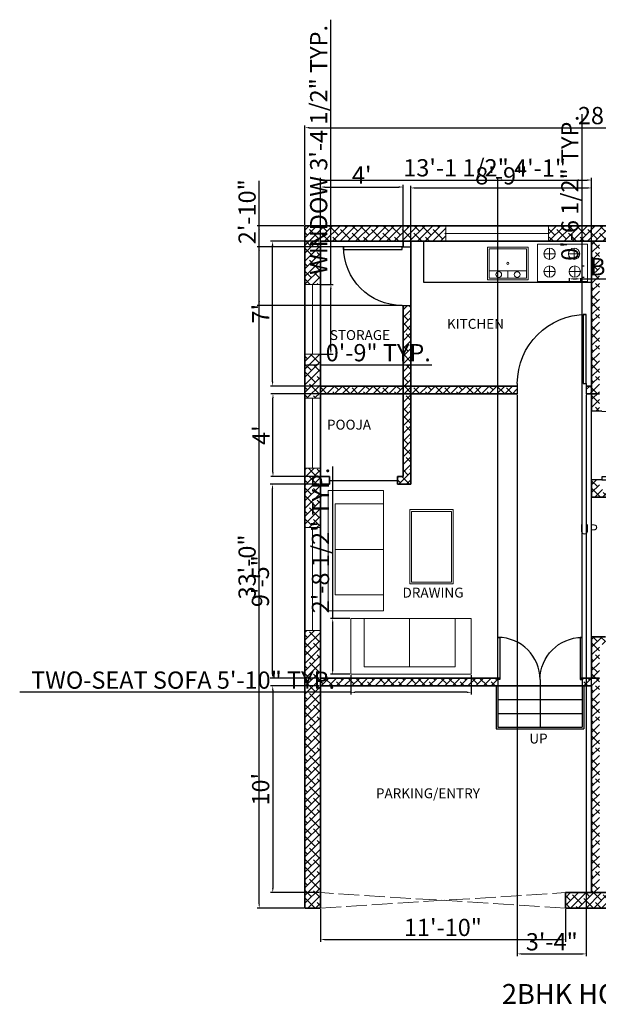
# Model space of a CAD drawing. Units: inches. Extents: x 1501 to 2163, y 1105 to 1729.
# Tile 1 of 2: x 1501 to 1837, y 1105 to 1676. Entities that reach past the tile are written whole.
import ezdxf

# ---------------------------------------------------------------- set-up
doc = ezdxf.new("R2010")
doc.units = ezdxf.units.IN
doc.linetypes.add('ACAD_ISO02W100', pattern=[15, 12, -3])
for name, color, linetype, lineweight in [('A-ANNO-DIMS', 2, 'Continuous', 18), ('A-ANNO-TEXT', 7, 'Continuous', 18), ('A-AREA-IDEN', 7, 'Continuous', 18), ('A-DOOR', 3, 'Continuous', 25), ('A-DOOR-OPEN', 3, 'ACAD_ISO02W100', 18), ('A-EQPM', 9, 'Continuous', 18), ('A-FLOR-CASE', 8, 'Continuous', 25), ('A-FLOR-FIXT', 9, 'Continuous', 18), ('A-FLOR-STRS', 7, 'Continuous', 25), ('A-GLAZ', 4, 'Continuous', 18), ('A-WALL', 7, 'Continuous', 35), ('A-WALL-PATT', 252, 'Continuous', 13), ('fur', 130, 'Continuous', 18)]:
    doc.layers.add(name, color=color, linetype=linetype, lineweight=lineweight)
doc.styles.get("Standard").update_dxf_attribs({"font": 'arial.ttf'})
doc.dimstyles.new('ISO-25', dxfattribs={"dimtxt": 10, "dimasz": 2.5, "dimexe": 1.25, "dimexo": 0.625, "dimtad": 1, "dimdec": 0, "dimlunit": 4, "dimtxsty": 'Standard', "dimcen": 2.5, "dimadec": 0, "dimazin": 0, "dimtfac": 1, "dimtdec": 0, "dimtmove": 0, "dimatfit": 3, "dimfxl": 1, "dimarcsym": 0})

# ---------------------------------------------------------------- blocks, each defined once
blk = doc.blocks.new('*U2')
for p, q in [((0, 0), (0, -6)), ((40, 0), (40, -6))]:
    blk.add_line(p, q)
blk.add_lwpolyline([(0, 0), (0, 40), (1.75, 40), (1.75, 0)], close=True)
blk.add_arc((0, 0), 40, 0, 90)
blk = doc.blocks.new('*D12')
at = {"layer": 'A-ANNO-DIMS', "color": 0, "lineweight": -2, "transparency": 16777216}
for p, q in [((1666.55, 1557.41), (1666.55, 1614.95)), ((1669.05, 1613.7), (2000.05, 1613.7)), ((2002.55, 1557.41), (2002.55, 1614.95))]:
    blk.add_line(p, q, dxfattribs=at)
at = {"layer": 'A-ANNO-DIMS', "color": 0, "lineweight": 100, "transparency": 16777216}
for points in [[(1669.05, 1614.12), (1669.05, 1613.29), (1666.55, 1613.7)], [(2000.05, 1614.12), (2000.05, 1613.29), (2002.55, 1613.7)]]:
    blk.add_solid(points, dxfattribs=at)
at = {"layer": 'Defpoints', "color": 0, "lineweight": 100, "transparency": 16777216}
for p in [(2002.55, 1613.7), (1666.55, 1556.78), (2002.55, 1556.78)]:
    blk.add_point(p, dxfattribs=at)
at = {"layer": 'A-ANNO-DIMS', "color": 0, "transparency": 16777216, "insert": (1834.55, 1619.44), "char_height": 10, "attachment_point": 5}
blk.add_mtext("28'", dxfattribs=at)
blk = doc.blocks.new('*D13')
at = {"layer": 'A-ANNO-DIMS', "color": 0, "lineweight": -2, "transparency": 16777216}
for p, q in [((1675.55, 1548.41), (1675.55, 1580.52)), ((1678.05, 1579.27), (1721.05, 1579.27)), ((1723.55, 1548.41), (1723.55, 1580.52))]:
    blk.add_line(p, q, dxfattribs=at)
at = {"layer": 'A-ANNO-DIMS', "color": 0, "lineweight": 100, "transparency": 16777216}
for points in [[(1678.05, 1579.69), (1678.05, 1578.85), (1675.55, 1579.27)], [(1721.05, 1579.69), (1721.05, 1578.85), (1723.55, 1579.27)]]:
    blk.add_solid(points, dxfattribs=at)
at = {"layer": 'Defpoints', "color": 0, "lineweight": 100, "transparency": 16777216}
for p in [(1723.55, 1579.27), (1675.55, 1547.78), (1723.55, 1547.78)]:
    blk.add_point(p, dxfattribs=at)
at = {"layer": 'A-ANNO-DIMS', "color": 0, "transparency": 16777216, "insert": (1699.55, 1584.89), "char_height": 10, "attachment_point": 5}
blk.add_mtext("4'", dxfattribs=at)
blk = doc.blocks.new('*D14')
at = {"layer": 'A-ANNO-DIMS', "color": 0, "lineweight": -2, "transparency": 16777216}
for p, q in [((1728.05, 1548.41), (1728.05, 1579.99)), ((1730.55, 1578.74), (1830.55, 1578.74)), ((1833.05, 1548.41), (1833.05, 1579.99))]:
    blk.add_line(p, q, dxfattribs=at)
at = {"layer": 'A-ANNO-DIMS', "color": 0, "lineweight": 100, "transparency": 16777216}
for points in [[(1730.55, 1579.15), (1730.55, 1578.32), (1728.05, 1578.74)], [(1830.55, 1579.15), (1830.55, 1578.32), (1833.05, 1578.74)]]:
    blk.add_solid(points, dxfattribs=at)
at = {"layer": 'Defpoints', "color": 0, "lineweight": 100, "transparency": 16777216}
for p in [(1833.05, 1578.74), (1728.05, 1547.78), (1833.05, 1547.78)]:
    blk.add_point(p, dxfattribs=at)
at = {"layer": 'A-ANNO-DIMS', "color": 0, "transparency": 16777216, "insert": (1780.55, 1584.47), "char_height": 10, "attachment_point": 5}
blk.add_mtext('8\'-9"', dxfattribs=at)
blk = doc.blocks.new('*D20')
at = {"layer": 'A-ANNO-DIMS', "color": 0, "lineweight": -2, "transparency": 16777216}
for p, q in [((1675.55, 1160.16), (1675.55, 1141.32)), ((1817.84, 1160.16), (1817.84, 1141.32)), ((1678.05, 1142.57), (1815.34, 1142.57))]:
    blk.add_line(p, q, dxfattribs=at)
at = {"layer": 'A-ANNO-DIMS', "color": 0, "lineweight": 100, "transparency": 16777216}
for points in [[(1678.05, 1142.98), (1678.05, 1142.15), (1675.55, 1142.57)], [(1815.34, 1142.98), (1815.34, 1142.15), (1817.84, 1142.57)]]:
    blk.add_solid(points, dxfattribs=at)
at = {"layer": 'Defpoints', "color": 0, "lineweight": 100, "transparency": 16777216}
for p in [(1675.55, 1160.78), (1817.84, 1160.78), (1817.84, 1142.57)]:
    blk.add_point(p, dxfattribs=at)
at = {"layer": 'A-ANNO-DIMS', "color": 0, "transparency": 16777216, "insert": (1746.69, 1148.3), "char_height": 10, "attachment_point": 5}
blk.add_mtext('11\'-10"', dxfattribs=at)
blk = doc.blocks.new('*D21')
at = {"layer": 'A-ANNO-DIMS', "color": 0, "lineweight": -2, "transparency": 16777216}
for p, q in [((1674.93, 1289.78), (1646.64, 1289.78)), ((1647.89, 1287.28), (1647.89, 1172.28)), ((1674.93, 1169.78), (1646.64, 1169.78))]:
    blk.add_line(p, q, dxfattribs=at)
at = {"layer": 'A-ANNO-DIMS', "color": 0, "lineweight": 100, "transparency": 16777216}
for points in [[(1647.47, 1287.28), (1648.3, 1287.28), (1647.89, 1289.78)], [(1647.47, 1172.28), (1648.3, 1172.28), (1647.89, 1169.78)]]:
    blk.add_solid(points, dxfattribs=at)
at = {"layer": 'Defpoints', "color": 0, "lineweight": 100, "transparency": 16777216}
for p in [(1675.55, 1289.78), (1647.89, 1169.78), (1675.55, 1169.78)]:
    blk.add_point(p, dxfattribs=at)
at = {"layer": 'A-ANNO-DIMS', "color": 0, "transparency": 16777216, "insert": (1642.15, 1229.78), "char_height": 10, "attachment_point": 5, "rotation": 90}
blk.add_mtext("10'", dxfattribs=at)
blk = doc.blocks.new('*D22')
at = {"layer": 'A-ANNO-DIMS', "color": 0, "lineweight": -2, "transparency": 16777216}
for p, q in [((1674.93, 1406.78), (1646.47, 1406.78)), ((1647.72, 1296.78), (1647.72, 1404.28)), ((1674.93, 1294.28), (1646.47, 1294.28))]:
    blk.add_line(p, q, dxfattribs=at)
at = {"layer": 'A-ANNO-DIMS', "color": 0, "lineweight": 100, "transparency": 16777216}
for points in [[(1647.31, 1404.28), (1648.14, 1404.28), (1647.72, 1406.78)], [(1647.31, 1296.78), (1648.14, 1296.78), (1647.72, 1294.28)]]:
    blk.add_solid(points, dxfattribs=at)
at = {"layer": 'Defpoints', "color": 0, "lineweight": 100, "transparency": 16777216}
for p in [(1647.72, 1406.78), (1675.55, 1406.78), (1675.55, 1294.28)]:
    blk.add_point(p, dxfattribs=at)
at = {"layer": 'A-ANNO-DIMS', "color": 0, "transparency": 16777216, "insert": (1641.99, 1350.53), "char_height": 10, "attachment_point": 5, "rotation": 90}
blk.add_mtext('9\'-5"', dxfattribs=at)
blk = doc.blocks.new('*D23')
at = {"layer": 'A-ANNO-DIMS', "color": 0, "lineweight": -2, "transparency": 16777216}
for p, q in [((1674.93, 1459.28), (1646.75, 1459.28)), ((1648, 1413.78), (1648, 1456.78)), ((1674.93, 1411.28), (1646.75, 1411.28))]:
    blk.add_line(p, q, dxfattribs=at)
at = {"layer": 'A-ANNO-DIMS', "color": 0, "lineweight": 100, "transparency": 16777216}
for points in [[(1647.59, 1456.78), (1648.42, 1456.78), (1648, 1459.28)], [(1647.59, 1413.78), (1648.42, 1413.78), (1648, 1411.28)]]:
    blk.add_solid(points, dxfattribs=at)
at = {"layer": 'Defpoints', "color": 0, "lineweight": 100, "transparency": 16777216}
for p in [(1648, 1459.28), (1675.55, 1459.28), (1675.55, 1411.28)]:
    blk.add_point(p, dxfattribs=at)
at = {"layer": 'A-ANNO-DIMS', "color": 0, "transparency": 16777216, "insert": (1642.38, 1435.28), "char_height": 10, "attachment_point": 5, "rotation": 90}
blk.add_mtext("4'", dxfattribs=at)
blk = doc.blocks.new('*D24')
at = {"layer": 'A-ANNO-DIMS', "color": 0, "lineweight": -2, "transparency": 16777216}
for p, q in [((1674.93, 1547.78), (1646.55, 1547.78)), ((1647.8, 1466.28), (1647.8, 1545.28)), ((1674.93, 1463.78), (1646.55, 1463.78))]:
    blk.add_line(p, q, dxfattribs=at)
at = {"layer": 'A-ANNO-DIMS', "color": 0, "lineweight": 100, "transparency": 16777216}
for points in [[(1647.38, 1545.28), (1648.21, 1545.28), (1647.8, 1547.78)], [(1647.38, 1466.28), (1648.21, 1466.28), (1647.8, 1463.78)]]:
    blk.add_solid(points, dxfattribs=at)
at = {"layer": 'Defpoints', "color": 0, "lineweight": 100, "transparency": 16777216}
for p in [(1647.8, 1547.78), (1675.55, 1547.78), (1675.55, 1463.78)]:
    blk.add_point(p, dxfattribs=at)
at = {"layer": 'A-ANNO-DIMS', "color": 0, "transparency": 16777216, "insert": (1642.17, 1505.78), "char_height": 10, "attachment_point": 5, "rotation": 90}
blk.add_mtext("7'", dxfattribs=at)
blk = doc.blocks.new('WIN-60IN')
blk.add_line((0, 4.5), (59.67, 4.5))
blk.add_lwpolyline([(0, 9), (59.67, 9), (59.67, 0), (0, 0)], close=True)
blk = doc.blocks.new('WIN-41IN')
blk.add_line((4.5, 0), (4.5, 40.59))
blk.add_lwpolyline([(0, 0), (9, 0), (9, 40.59), (0, 40.59)], close=True)
blk = doc.blocks.new('SOFA-TWO-SEAT')
for p, q in [((32.31, 69.96), (0, 69.96)), ((0, 69.96), (0, 0)), ((32.31, 62.16), (32.31, 69.96)), ((4.25, 35.75), (32.31, 35.75)), ((32.31, 0), (32.31, 9.35)), ((0, 0), (32.31, 0))]:
    blk.add_line(p, q)
blk.add_lwpolyline([(4.25, 62.16), (32.31, 62.16), (32.31, 9.35), (4.25, 9.35)], close=True)
blk = doc.blocks.new('COOKTOP-BURNER')
for p, q in [((3.26, 6.53), (3.26, 0)), ((6.53, 3.27), (0, 3.27)), ((3.26, 0), (3.26, 3.27)), ((3.26, 3.27), (6.53, 3.27))]:
    blk.add_line(p, q)
blk.add_circle((3.26, 3.27), 3.26)
blk = doc.blocks.new('*D34')
at = {"layer": 'A-ANNO-DIMS', "color": 0, "lineweight": -2, "transparency": 16777216}
for p, q in [((1681.64, 1522.79), (1681.64, 1676.38)), ((1676.18, 1522.79), (1682.89, 1522.79)), ((1681.64, 1484.69), (1681.64, 1520.29)), ((1676.18, 1482.19), (1682.89, 1482.19))]:
    blk.add_line(p, q, dxfattribs=at)
at = {"layer": 'A-ANNO-DIMS', "color": 0, "lineweight": 100, "transparency": 16777216}
for points in [[(1681.22, 1520.29), (1682.06, 1520.29), (1681.64, 1522.79)], [(1681.22, 1484.69), (1682.06, 1484.69), (1681.64, 1482.19)]]:
    blk.add_solid(points, dxfattribs=at)
at = {"layer": 'Defpoints', "color": 0, "lineweight": 100, "transparency": 16777216}
for p in [(1675.55, 1522.79), (1681.64, 1522.79), (1675.55, 1482.19)]:
    blk.add_point(p, dxfattribs=at)
at = {"layer": 'A-ANNO-DIMS', "color": 0, "transparency": 16777216, "insert": (1675.84, 1600.83), "char_height": 10, "attachment_point": 5, "rotation": 90}
blk.add_mtext('WINDOW 3\'-4 1/2" TYP.', dxfattribs=at)
blk = doc.blocks.new('*D35')
at = {"layer": 'A-ANNO-DIMS', "color": 0, "lineweight": -2, "transparency": 16777216}
for p, q in [((1666.55, 1481.57), (1666.55, 1474.86)), ((1675.55, 1481.57), (1675.55, 1474.86)), ((1669.05, 1476.11), (1673.05, 1476.11)), ((1675.55, 1476.11), (1740.26, 1476.11))]:
    blk.add_line(p, q, dxfattribs=at)
at = {"layer": 'A-ANNO-DIMS', "color": 0, "lineweight": 100, "transparency": 16777216}
for points in [[(1669.05, 1476.52), (1669.05, 1475.69), (1666.55, 1476.11)], [(1673.05, 1476.52), (1673.05, 1475.69), (1675.55, 1476.11)]]:
    blk.add_solid(points, dxfattribs=at)
at = {"layer": 'Defpoints', "color": 0, "lineweight": 100, "transparency": 16777216}
for p in [(1666.55, 1482.19), (1675.55, 1482.19), (1675.55, 1476.11)]:
    blk.add_point(p, dxfattribs=at)
at = {"layer": 'A-ANNO-DIMS', "color": 0, "transparency": 16777216, "insert": (1709.15, 1481.84), "char_height": 10, "attachment_point": 5}
blk.add_mtext('0\'-9" TYP.', dxfattribs=at)
blk = doc.blocks.new('*D36')
at = {"layer": 'A-ANNO-DIMS', "color": 0, "lineweight": -2, "transparency": 16777216}
for p, q in [((1693.17, 1295.9), (1693.17, 1284.78)), ((1763.13, 1295.9), (1763.13, 1284.78)), ((1693.17, 1286.03), (1500.92, 1286.03)), ((1760.63, 1286.03), (1695.67, 1286.03))]:
    blk.add_line(p, q, dxfattribs=at)
at = {"layer": 'A-ANNO-DIMS', "color": 0, "lineweight": 100, "transparency": 16777216}
for points in [[(1695.67, 1286.44), (1695.67, 1285.61), (1693.17, 1286.03)], [(1760.63, 1286.44), (1760.63, 1285.61), (1763.13, 1286.03)]]:
    blk.add_solid(points, dxfattribs=at)
at = {"layer": 'Defpoints', "color": 0, "lineweight": 100, "transparency": 16777216}
for p in [(1693.17, 1296.52), (1763.13, 1296.52), (1693.17, 1286.03)]:
    blk.add_point(p, dxfattribs=at)
at = {"layer": 'A-ANNO-DIMS', "color": 0, "transparency": 16777216, "insert": (1595.8, 1291.83), "char_height": 10, "attachment_point": 5}
blk.add_mtext('TWO-SEAT SOFA 5\'-10" TYP.', dxfattribs=at)
blk = doc.blocks.new('*D37')
at = {"layer": 'A-ANNO-DIMS', "color": 0, "lineweight": -2, "transparency": 16777216}
for p, q in [((1682.68, 1328.83), (1682.68, 1417.01)), ((1692.55, 1328.83), (1681.43, 1328.83)), ((1682.68, 1299.02), (1682.68, 1326.33)), ((1692.55, 1296.52), (1681.43, 1296.52))]:
    blk.add_line(p, q, dxfattribs=at)
at = {"layer": 'A-ANNO-DIMS', "color": 0, "lineweight": 100, "transparency": 16777216}
for points in [[(1682.26, 1326.33), (1683.1, 1326.33), (1682.68, 1328.83)], [(1682.26, 1299.02), (1683.1, 1299.02), (1682.68, 1296.52)]]:
    blk.add_solid(points, dxfattribs=at)
at = {"layer": 'Defpoints', "color": 0, "lineweight": 100, "transparency": 16777216}
for p in [(1682.68, 1328.83), (1693.17, 1328.83), (1693.17, 1296.52)]:
    blk.add_point(p, dxfattribs=at)
at = {"layer": 'A-ANNO-DIMS', "color": 0, "transparency": 16777216, "insert": (1676.88, 1374.17), "char_height": 10, "attachment_point": 5, "rotation": 90}
blk.add_mtext('2\'-8 1/2" TYP.', dxfattribs=at)
blk = doc.blocks.new('*D44')
at = {"layer": 'A-ANNO-DIMS', "color": 0, "lineweight": -2, "transparency": 16777216}
for p, q in [((1820, 1526.33), (1820, 1524.73)), ((1822.5, 1525.98), (1824.03, 1525.98)), ((1826.53, 1526.33), (1826.53, 1524.73)), ((1826.53, 1525.98), (1976.97, 1525.98))]:
    blk.add_line(p, q, dxfattribs=at)
at = {"layer": 'A-ANNO-DIMS', "color": 0, "lineweight": 100, "transparency": 16777216}
for points in [[(1822.5, 1526.39), (1822.5, 1525.56), (1820, 1525.98)], [(1824.03, 1526.39), (1824.03, 1525.56), (1826.53, 1525.98)]]:
    blk.add_solid(points, dxfattribs=at)
at = {"layer": 'Defpoints', "color": 0, "lineweight": 100, "transparency": 16777216}
for p in [(1820, 1526.95), (1826.53, 1526.95), (1826.53, 1525.98)]:
    blk.add_point(p, dxfattribs=at)
at = {"layer": 'A-ANNO-DIMS', "color": 0, "transparency": 16777216, "insert": (1903, 1531.77), "char_height": 10, "attachment_point": 5}
blk.add_mtext('BURNER 0\'-6 1/2" TYP.', dxfattribs=at)
blk = doc.blocks.new('*D45')
at = {"layer": 'A-ANNO-DIMS', "color": 0, "lineweight": -2, "transparency": 16777216}
for p, q in [((1827.51, 1533.48), (1827.51, 1621.49)), ((1827.16, 1533.48), (1828.76, 1533.48)), ((1827.16, 1526.95), (1828.76, 1526.95)), ((1827.51, 1529.45), (1827.51, 1530.98))]:
    blk.add_line(p, q, dxfattribs=at)
at = {"layer": 'A-ANNO-DIMS', "color": 0, "lineweight": 100, "transparency": 16777216}
for points in [[(1827.1, 1530.98), (1827.93, 1530.98), (1827.51, 1533.48)], [(1827.1, 1529.45), (1827.93, 1529.45), (1827.51, 1526.95)]]:
    blk.add_solid(points, dxfattribs=at)
at = {"layer": 'Defpoints', "color": 0, "lineweight": 100, "transparency": 16777216}
for p in [(1826.53, 1533.48), (1827.51, 1533.48), (1826.53, 1526.95)]:
    blk.add_point(p, dxfattribs=at)
at = {"layer": 'A-ANNO-DIMS', "color": 0, "transparency": 16777216, "insert": (1821.72, 1578.74), "char_height": 10, "attachment_point": 5, "rotation": 90}
blk.add_mtext('0\'-6 1/2" TYP.', dxfattribs=at)
blk = doc.blocks.new('*D46')
at = {"layer": 'A-ANNO-DIMS', "color": 0, "lineweight": -2, "transparency": 16777216}
for p, q in [((1665.93, 1556.78), (1638.75, 1556.78)), ((1640, 1163.28), (1640, 1554.28)), ((1665.93, 1160.78), (1638.75, 1160.78))]:
    blk.add_line(p, q, dxfattribs=at)
at = {"layer": 'A-ANNO-DIMS', "color": 0, "lineweight": 100, "transparency": 16777216}
for points in [[(1639.58, 1554.28), (1640.42, 1554.28), (1640, 1556.78)], [(1639.58, 1163.28), (1640.42, 1163.28), (1640, 1160.78)]]:
    blk.add_solid(points, dxfattribs=at)
at = {"layer": 'Defpoints', "color": 0, "lineweight": 100, "transparency": 16777216}
for p in [(1640, 1556.78), (1666.55, 1556.78), (1666.55, 1160.78)]:
    blk.add_point(p, dxfattribs=at)
at = {"layer": 'A-ANNO-DIMS', "color": 0, "transparency": 16777216, "insert": (1634.27, 1358.78), "char_height": 10, "attachment_point": 5, "rotation": 90}
blk.add_mtext('33\'-0"', dxfattribs=at)
blk = doc.blocks.new('*D47')
at = {"layer": 'A-ANNO-DIMS', "color": 0, "lineweight": -2, "transparency": 16777216}
for p, q in [((1778.68, 1294.07), (1778.68, 1584.58)), ((1781.18, 1583.33), (1825.03, 1583.33)), ((1827.53, 1294.07), (1827.53, 1584.58))]:
    blk.add_line(p, q, dxfattribs=at)
at = {"layer": 'A-ANNO-DIMS', "color": 0, "lineweight": 100, "transparency": 16777216}
for points in [[(1781.18, 1583.75), (1781.18, 1582.92), (1778.68, 1583.33)], [(1825.03, 1583.75), (1825.03, 1582.92), (1827.53, 1583.33)]]:
    blk.add_solid(points, dxfattribs=at)
at = {"layer": 'Defpoints', "color": 0, "lineweight": 100, "transparency": 16777216}
for p in [(1827.53, 1583.33), (1778.68, 1293.45), (1827.53, 1293.45)]:
    blk.add_point(p, dxfattribs=at)
at = {"layer": 'A-ANNO-DIMS', "color": 0, "transparency": 16777216, "insert": (1803.1, 1588.98), "char_height": 10, "attachment_point": 5}
blk.add_mtext('4\'-1"', dxfattribs=at)
blk = doc.blocks.new('*D48')
at = {"layer": 'A-ANNO-DIMS', "color": 0, "lineweight": -2, "transparency": 16777216}
for p, q in [((1789.9, 1458.66), (1789.9, 1132.98)), ((1829.9, 1458.66), (1829.9, 1132.98)), ((1792.4, 1134.23), (1827.4, 1134.23))]:
    blk.add_line(p, q, dxfattribs=at)
at = {"layer": 'A-ANNO-DIMS', "color": 0, "lineweight": 100, "transparency": 16777216}
for points in [[(1792.4, 1134.65), (1792.4, 1133.82), (1789.9, 1134.23)], [(1827.4, 1134.65), (1827.4, 1133.82), (1829.9, 1134.23)]]:
    blk.add_solid(points, dxfattribs=at)
at = {"layer": 'Defpoints', "color": 0, "lineweight": 100, "transparency": 16777216}
for p in [(1789.9, 1459.28), (1829.9, 1459.28), (1829.9, 1134.23)]:
    blk.add_point(p, dxfattribs=at)
at = {"layer": 'A-ANNO-DIMS', "color": 0, "transparency": 16777216, "insert": (1809.9, 1139.97), "char_height": 10, "attachment_point": 5}
blk.add_mtext('3\'-4"', dxfattribs=at)
blk = doc.blocks.new('*D49')
at = {"layer": 'A-ANNO-DIMS', "color": 0, "lineweight": -2, "transparency": 16777216}
for p, q in [((1640, 1544.56), (1640, 1582.83)), ((1722.93, 1544.56), (1638.75, 1544.56)), ((1640, 1513.06), (1640, 1542.06)), ((1722.93, 1510.56), (1638.75, 1510.56))]:
    blk.add_line(p, q, dxfattribs=at)
at = {"layer": 'A-ANNO-DIMS', "color": 0, "lineweight": 100, "transparency": 16777216}
for points in [[(1639.58, 1542.06), (1640.42, 1542.06), (1640, 1544.56)], [(1639.58, 1513.06), (1640.42, 1513.06), (1640, 1510.56)]]:
    blk.add_solid(points, dxfattribs=at)
at = {"layer": 'Defpoints', "color": 0, "lineweight": 100, "transparency": 16777216}
for p in [(1640, 1544.56), (1723.55, 1544.56), (1723.55, 1510.56)]:
    blk.add_point(p, dxfattribs=at)
at = {"layer": 'A-ANNO-DIMS', "color": 0, "transparency": 16777216, "insert": (1634.27, 1564.94), "char_height": 10, "attachment_point": 5, "rotation": 90}
blk.add_mtext('2\'-10"', dxfattribs=at)
blk = doc.blocks.new('*D50')
at = {"layer": 'A-ANNO-DIMS', "color": 0, "lineweight": -2, "transparency": 16777216}
for p, q in [((1675.55, 1170.41), (1675.55, 1584.58)), ((1678.05, 1583.33), (1830.55, 1583.33)), ((1833.05, 1170.41), (1833.05, 1584.58))]:
    blk.add_line(p, q, dxfattribs=at)
at = {"layer": 'A-ANNO-DIMS', "color": 0, "lineweight": 100, "transparency": 16777216}
for points in [[(1678.05, 1583.75), (1678.05, 1582.92), (1675.55, 1583.33)], [(1830.55, 1583.75), (1830.55, 1582.92), (1833.05, 1583.33)]]:
    blk.add_solid(points, dxfattribs=at)
at = {"layer": 'Defpoints', "color": 0, "lineweight": 100, "transparency": 16777216}
for p in [(1833.05, 1583.33), (1675.55, 1169.78), (1833.05, 1169.78)]:
    blk.add_point(p, dxfattribs=at)
at = {"layer": 'A-ANNO-DIMS', "color": 0, "transparency": 16777216, "insert": (1754.3, 1589.13), "char_height": 10, "attachment_point": 5}
blk.add_mtext('13\'-1 1/2"', dxfattribs=at)

msp = doc.modelspace()

# ---------------------------------------------------------------- hatches: boundary and pattern name
at = {"layer": 'A-WALL-PATT'}
h = msp.add_hatch(dxfattribs=at)
h.set_pattern_fill('ANSI38', color=256)
h.paths.add_polyline_path([(1748.43, 1556.78), (1666.55, 1556.78), (1666.55, 1522.79), (1675.55, 1522.79), (1675.55, 1547.78), (1748.43, 1547.78)])
h.paths.add_polyline_path([(1880.88, 1556.78), (1808.1, 1556.78), (1808.1, 1547.78), (1880.88, 1547.78)])
h.paths.add_polyline_path([(2002.55, 1556.78), (1940.55, 1556.78), (1940.55, 1547.78), (1993.55, 1547.78), (1993.55, 1502.88), (2002.55, 1502.88)])
h.paths.add_polyline_path([(1675.55, 1482.19), (1666.55, 1482.19), (1666.55, 1456.67), (1675.55, 1456.67)])
h.paths.add_polyline_path([(1675.55, 1321.98), (1666.55, 1321.98), (1666.55, 1160.78), (1675.55, 1160.78), (1675.55, 1169.78)])
h.paths.add_polyline_path([(1778.68, 1293.45), (1778.68, 1294.28), (1675.55, 1294.28), (1675.55, 1289.78), (1778.68, 1289.78)])
h.paths.add_polyline_path([(1675.55, 1406.78), (1675.55, 1416.08), (1666.55, 1416.08), (1666.55, 1381.65), (1675.55, 1381.65)])
h = msp.add_hatch(dxfattribs=at)
h.set_pattern_fill('ANSI38', color=256)
h.paths.add_polyline_path([(1728.05, 1510.56), (1723.55, 1510.56), (1723.55, 1463.78), (1728.05, 1463.78)])
h.paths.add_polyline_path([(1728.05, 1463.28), (1728.05, 1463.78), (1723.55, 1463.78), (1675.55, 1463.78), (1675.55, 1459.28), (1728.05, 1459.28)])
h.paths.add_polyline_path([(1728.05, 1459.28), (1723.55, 1459.28), (1723.55, 1415.28), (1723.55, 1411.28), (1720.31, 1411.28), (1720.31, 1406.78), (1728.05, 1406.78)])
h.paths.add_polyline_path([(1789.9, 1463.78), (1728.05, 1463.78), (1728.05, 1463.28), (1728.05, 1459.28), (1789.9, 1459.28)])
h.paths.add_polyline_path([(1837.55, 1547.78), (1833.05, 1547.78), (1833.05, 1523.78), (1833.05, 1459.28), (1837.55, 1459.28)])
h.paths.add_polyline_path([(1833.05, 1463.78), (1829.9, 1463.78), (1829.9, 1459.28), (1833.05, 1459.28)])
h.paths.add_polyline_path([(1837.55, 1459.28), (1833.05, 1459.28), (1833.05, 1449.28), (1837.55, 1449.28)])
h.paths.add_polyline_path([(2002.55, 1443.21), (1993.55, 1443.21), (1993.55, 1379.58), (2002.55, 1379.58)])
h.paths.add_polyline_path([(2002.55, 1338.99), (1993.55, 1338.99), (1993.55, 1270.9), (2002.55, 1270.9)])
h.paths.add_polyline_path([(1993.55, 1318.28), (1957.55, 1318.28), (1881.07, 1318.28), (1881.07, 1313.78), (1993.55, 1313.78)])
h.paths.add_polyline_path([(2002.55, 1211.23), (1993.55, 1211.23), (1993.55, 1169.78), (1940.55, 1169.78), (1940.55, 1160.78), (2002.55, 1160.78)])
h.paths.add_polyline_path([(1880.88, 1169.78), (1817.84, 1169.78), (1817.84, 1160.78), (1880.88, 1160.78)])
h = msp.add_hatch(dxfattribs=at)
h.set_pattern_fill('ANSI38', color=256)
h.paths.add_polyline_path([(1993.55, 1403.78), (1870.74, 1403.78), (1837.55, 1403.78), (1837.55, 1409.28), (1833.05, 1409.28), (1833.05, 1399.28), (1993.55, 1399.28)])
h.paths.add_polyline_path([(1837.55, 1294.28), (1827.53, 1294.28), (1827.53, 1293.45), (1827.53, 1289.78), (1833.05, 1289.78), (1833.05, 1169.78), (1837.55, 1169.78)])
h.paths.add_polyline_path([(1837.55, 1313.78), (1841.07, 1313.78), (1841.07, 1318.28), (1833.05, 1318.28), (1833.05, 1294.28), (1837.55, 1294.28)])

# ---------------------------------------------------------------- linework, layer by layer
at = {"layer": 'A-DOOR'}
msp.add_line((1680.87, 1409.03), (1720.31, 1409.03), dxfattribs=at)
at = {"layer": 'A-DOOR-OPEN'}
for p, q in [((1675.55, 1160.78), (1817.84, 1169.78)), ((1817.84, 1160.78), (1675.55, 1169.78))]:
    msp.add_line(p, q, dxfattribs=at)
at = {"layer": 'A-EQPM'}
msp.add_lwpolyline([(1830.59, 1546.16), (1801.71, 1546.16), (1801.71, 1524.53), (1830.59, 1524.53)], close=True, dxfattribs=at)
at = {"layer": 'A-FLOR-CASE'}
for p, q in [((1735.55, 1523.78), (1735.55, 1547.78)), ((1833.05, 1547.78), (1833.05, 1523.78)), ((1833.05, 1523.78), (1735.55, 1523.78))]:
    msp.add_line(p, q, dxfattribs=at)
at = {"layer": 'A-FLOR-FIXT'}
for p, q in [((1773.53, 1530.67), (1795.25, 1530.67)), ((1784.39, 1526.46), (1784.39, 1530.67))]:
    msp.add_line(p, q, dxfattribs=at)
for points in [[(1796.25, 1544.39), (1772.53, 1544.39), (1772.53, 1525.46), (1796.25, 1525.46)], [(1795.25, 1543.39), (1773.53, 1543.39), (1773.53, 1526.46), (1795.25, 1526.46)]]:
    msp.add_lwpolyline(points, close=True, dxfattribs=at)
for centre, radius in [((1784.39, 1534.92), 0.648), ((1779.11, 1528.49), 1.68), ((1789.8, 1528.45), 1.68)]:
    msp.add_circle(centre, radius, dxfattribs=at)
at = {"layer": 'A-FLOR-STRS'}
for p, q in [((1777.68, 1289.78), (1777.68, 1264.78)), ((1778.68, 1289.78), (1827.53, 1289.78)), ((1778.68, 1289.78), (1778.68, 1265.78)), ((1803.1, 1289.78), (1803.1, 1265.78)), ((1827.53, 1289.78), (1827.53, 1265.78)), ((1828.53, 1289.78), (1828.53, 1264.78)), ((1778.68, 1281.78), (1827.53, 1281.78)), ((1778.68, 1273.78), (1827.53, 1273.78)), ((1777.68, 1264.78), (1828.53, 1264.78)), ((1778.68, 1265.78), (1827.53, 1265.78))]:
    msp.add_line(p, q, dxfattribs=at)
at = {"layer": 'A-WALL'}
for p, q in [((1666.55, 1556.78), (2002.55, 1556.78)), ((1666.55, 1160.78), (1666.55, 1556.78)), ((1675.55, 1547.78), (1723.55, 1547.78)), ((1723.55, 1547.78), (1723.55, 1544.56)), ((1728.05, 1547.78), (1728.05, 1459.28)), ((1728.05, 1547.78), (1812.05, 1547.78)), ((1812.05, 1547.78), (1833.05, 1547.78)), ((1833.05, 1547.78), (1833.05, 1463.78)), ((1833.05, 1547.78), (1833.05, 1449.28)), ((1723.55, 1510.56), (1723.55, 1463.78)), ((1723.55, 1463.78), (1675.55, 1463.78)), ((1789.9, 1463.78), (1723.55, 1463.78)), ((1723.55, 1415.28), (1723.55, 1463.28)), ((1728.05, 1406.78), (1728.05, 1463.28)), ((1833.05, 1463.78), (1829.9, 1463.78)), ((1728.05, 1459.28), (1675.55, 1459.28)), ((1675.55, 1459.28), (1675.55, 1411.28)), ((1789.9, 1459.28), (1723.55, 1459.28)), ((1837.55, 1459.28), (1829.9, 1459.28)), ((1723.55, 1411.28), (1723.55, 1415.28)), ((1675.55, 1411.28), (1680.87, 1411.28)), ((1675.55, 1406.78), (1680.87, 1406.78)), ((1675.55, 1406.78), (1675.55, 1241.78)), ((1675.55, 1406.78), (1675.55, 1250.78)), ((1675.55, 1406.78), (1675.55, 1294.28)), ((1680.87, 1406.78), (1680.87, 1411.28)), ((1720.31, 1411.28), (1720.31, 1406.78)), ((1720.31, 1411.28), (1723.55, 1411.28)), ((1720.31, 1406.78), (1728.05, 1406.78)), ((1833.05, 1409.28), (1833.05, 1399.28)), ((1833.05, 1399.28), (1993.55, 1399.28)), ((1833.05, 1294.28), (1833.05, 1318.28)), ((1841.07, 1318.28), (1833.05, 1318.28)), ((1675.55, 1294.28), (1779.74, 1294.28)), ((1803.09, 1294.28), (1803.12, 1294.28)), ((1826.46, 1294.28), (1837.55, 1294.28)), ((1675.55, 1289.78), (1833.05, 1289.78)), ((1833.05, 1169.78), (1833.05, 1289.78)), ((1675.55, 1169.78), (1675.55, 1160.78)), ((1817.84, 1169.78), (1833.05, 1169.78)), ((1817.84, 1169.78), (1817.84, 1160.78)), ((1675.55, 1160.78), (1666.55, 1160.78)), ((2002.55, 1160.78), (1817.84, 1160.78))]:
    msp.add_line(p, q, dxfattribs=at)
for points in [[(1675.55, 1160.78), (1666.55, 1160.78), (1666.55, 1556.78), (2002.55, 1556.78), (2002.55, 1160.78), (1817.84, 1160.78)], [(1675.55, 1169.78), (1675.55, 1547.78), (1993.55, 1547.78), (1993.55, 1169.78), (1817.84, 1169.78)]]:
    msp.add_lwpolyline(points, dxfattribs=at)
at = {"layer": 'fur'}
for points in [[(1727.49, 1348.96), (1752.67, 1348.96), (1752.67, 1392.04), (1727.49, 1392.04)], [(1728.49, 1349.96), (1751.67, 1349.96), (1751.67, 1391.04), (1728.49, 1391.04)]]:
    msp.add_lwpolyline(points, close=True, dxfattribs=at)

# ---------------------------------------------------------------- block references
at = {"layer": 'A-DOOR', "xscale": -0.8498138110531805, "yscale": 0.8498138110531805, "zscale": 0.8498138110531805, "rotation": 90}
msp.add_blockref('*U2', (1722.95, 1544.56), dxfattribs=at)
at = {"layer": 'A-DOOR', "xscale": -1}
msp.add_blockref('*U2', (1829.9, 1465.28), dxfattribs=at)
at = {"layer": 'A-DOOR', "xscale": -1, "rotation": 270}
msp.add_blockref('*U2', (1839.05, 1409.28), dxfattribs=at)
at = {"layer": 'A-DOOR', "yscale": 0.610687977208717, "zscale": 0.610687977208717}
for p, xscale in [((1778.68, 1293.45), 0.610687977208717), ((1827.53, 1293.45), -0.610687977208717)]:
    msp.add_blockref('*U2', p, dxfattribs=dict(at, xscale=xscale))
at = {"layer": 'A-EQPM'}
for p in [(1805.34, 1537.24), (1819.59, 1537.24), (1805.34, 1526.95), (1820, 1526.95)]:
    msp.add_blockref('COOKTOP-BURNER', p, dxfattribs=at)
at = {"layer": 'A-GLAZ'}
for name, p in [('WIN-60IN', (1748.43, 1547.79)), ('WIN-41IN', (1666.55, 1482.19)), ('WIN-41IN', (1666.55, 1416.08))]:
    msp.add_blockref(name, p, dxfattribs=at)
at = {"layer": 'A-GLAZ', "rotation": 269.9999999999993}
msp.add_blockref('WIN-60IN', (1666.55, 1381.65), dxfattribs=at)
at = {"layer": 'fur'}
msp.add_blockref('SOFA-TWO-SEAT', (1679.97, 1333.23), dxfattribs=at)
at = {"layer": 'fur', "rotation": 89.99999999999928}
msp.add_blockref('SOFA-TWO-SEAT', (1763.13, 1296.52), dxfattribs=at)

# ---------------------------------------------------------------- texts
at = {"layer": 'A-ANNO-TEXT', "attachment_point": 1}
for s, width, gutter_width, insert, char_height in [('UP', 61.1637, 28.76, (1826.08, 1383.47), 5.753), ('UP', 61.1637, 28.76, (1796.87, 1262.09), 5.753), ('2BHK HOUSE PLAN', 1377.2449, 57.83, (1780.96, 1116.75), 11.5661)]:
    msp.add_mtext_dynamic_manual_height_columns(s, width=width, gutter_width=gutter_width, heights=[0], dxfattribs=dict(at, insert=insert, char_height=char_height))
at = {"layer": 'A-AREA-IDEN', "attachment_point": 1}
for s, insert, char_height in [('KITCHEN', (1749.04, 1502.73), 5.753), ('STORAGE', (1681.03, 1496.24), 5.753), ('POOJA', (1679.36, 1444.23), 5.753), ('DRAWING', (1723.24, 1346.77), 5.753), ('PARKING/ENTRY', (1707.79, 1230.3), 5.7528)]:
    msp.add_mtext_dynamic_manual_height_columns(s, width=61.1637, gutter_width=28.76, heights=[0], dxfattribs=dict(at, insert=insert, char_height=char_height))

# ---------------------------------------------------------------- dimensions: what is measured, and where the dimension line sits
at = {"layer": 'A-ANNO-DIMS'}
for base, p1, p2, angle, text, picture, middle in [((1681.64, 1522.79), (1675.55, 1482.19), (1675.55, 1522.79), 90, 'WINDOW <> TYP.', '*D34', (1675.84, 1600.83)), ((1827.51, 1533.48), (1826.53, 1526.95), (1826.53, 1533.48), 90, '<> TYP.', '*D45', (1821.72, 1578.74)), ((1682.68, 1328.83), (1693.17, 1296.52), (1693.17, 1328.83), 90, '<> TYP.', '*D37', (1676.88, 1374.17)), ((1693.17, 1286.03), (1763.13, 1296.52), (1693.17, 1296.52), 180, 'TWO-SEAT SOFA <> TYP.', '*D36', (1595.8, 1291.83))]:
    dim = msp.add_linear_dim(base=base, p1=p1, p2=p2, angle=angle, text=text, dimstyle='ISO-25', override={"dimdec": 1, "dimlfac": 1, "dimrnd": 0, "dimzin": 1, "dimdsep": 46, "dimlunit": 4, "dimfrac": 2}, dxfattribs=at)
    dim.commit()
    dim.dimension.update_dxf_attribs({"geometry": picture, "text_midpoint": middle})
for base, p1, p2, override, picture, middle in [((2002.55, 1613.7), (1666.55, 1556.78), (2002.55, 1556.78), {"dimclrd": 0, "dimclre": 0, "dimclrt": 0}, '*D12', (1834.55, 1619.44)), ((1833.05, 1583.33), (1675.55, 1169.78), (1833.05, 1169.78), {"dimdec": 1, "dimlfac": 1, "dimrnd": 0, "dimzin": 1, "dimdsep": 46, "dimlunit": 4, "dimfrac": 2}, '*D50', (1754.3, 1589.13)), ((1827.5309, 1583.3348), (1778.6758, 1293.4489), (1827.5309, 1293.4489), {"dimdec": 1, "dimlfac": 1, "dimrnd": 0, "dimzin": 1, "dimdsep": 46, "dimlunit": 4, "dimfrac": 2}, '*D47', (1803.1033, 1588.9802)), ((1723.55, 1579.27), (1675.55, 1547.78), (1723.55, 1547.78), {"dimclrd": 0, "dimclre": 0, "dimclrt": 0}, '*D13', (1699.55, 1584.89)), ((1833.05, 1578.74), (1728.05, 1547.78), (1833.05, 1547.78), {"dimclrd": 0, "dimclre": 0, "dimclrt": 0}, '*D14', (1780.55, 1584.47)), ((1829.9, 1134.23), (1789.9, 1459.28), (1829.9, 1459.28), {"dimdec": 1, "dimlfac": 1, "dimrnd": 0, "dimzin": 1, "dimdsep": 46, "dimlunit": 4, "dimfrac": 2}, '*D48', (1809.9, 1139.97)), ((1817.84, 1142.57), (1675.55, 1160.78), (1817.84, 1160.78), {"dimclrd": 0, "dimclre": 0, "dimclrt": 0}, '*D20', (1746.69, 1148.3))]:
    dim = msp.add_linear_dim(base=base, p1=p1, p2=p2, dimstyle='ISO-25', override=override, dxfattribs=at)
    dim.commit()
    dim.dimension.update_dxf_attribs({"geometry": picture, "text_midpoint": middle})
for base, p1, p2, override, picture, middle in [((1640, 1544.56), (1723.55, 1510.56), (1723.55, 1544.56), {"dimdec": 1, "dimlfac": 1, "dimrnd": 0, "dimzin": 1, "dimdsep": 46, "dimlunit": 4, "dimfrac": 2}, '*D49', (1634.27, 1564.94)), ((1640, 1556.78), (1666.55, 1160.78), (1666.55, 1556.78), {"dimdec": 1, "dimlfac": 1, "dimrnd": 0, "dimzin": 1, "dimdsep": 46, "dimlunit": 4, "dimfrac": 2}, '*D46', (1634.27, 1358.78)), ((1647.8, 1547.78), (1675.55, 1463.78), (1675.55, 1547.78), {"dimclrd": 0, "dimclre": 0, "dimclrt": 0}, '*D24', (1642.17, 1505.78)), ((1648, 1459.28), (1675.55, 1411.28), (1675.55, 1459.28), {"dimclrd": 0, "dimclre": 0, "dimclrt": 0}, '*D23', (1642.38, 1435.28)), ((1647.7219563, 1406.78475918), (1675.55075794, 1294.28475918), (1675.55075794, 1406.78475918), {"dimclrd": 0, "dimclre": 0, "dimclrt": 0}, '*D22', (1641.99122642, 1350.53475918)), ((1647.89, 1169.78), (1675.55, 1289.78), (1675.55, 1169.78), {"dimclrd": 0, "dimclre": 0, "dimclrt": 0}, '*D21', (1642.15, 1229.78))]:
    dim = msp.add_linear_dim(base=base, p1=p1, p2=p2, angle=90, dimstyle='ISO-25', override=override, dxfattribs=at)
    dim.commit()
    dim.dimension.update_dxf_attribs({"geometry": picture, "text_midpoint": middle})
for base, p1, p2, text, picture, middle in [((1826.53, 1525.98), (1820, 1526.95), (1826.53, 1526.95), 'BURNER <> TYP.', '*D44', (1903, 1531.77)), ((1675.55, 1476.11), (1666.55, 1482.19), (1675.55, 1482.19), '<> TYP.', '*D35', (1709.15, 1481.84))]:
    dim = msp.add_linear_dim(base=base, p1=p1, p2=p2, text=text, dimstyle='ISO-25', override={"dimdec": 1, "dimlfac": 1, "dimrnd": 0, "dimzin": 1, "dimdsep": 46, "dimlunit": 4, "dimfrac": 2}, dxfattribs=at)
    dim.commit()
    dim.dimension.update_dxf_attribs({"geometry": picture, "text_midpoint": middle})

doc.saveas('drawing.dxf')
